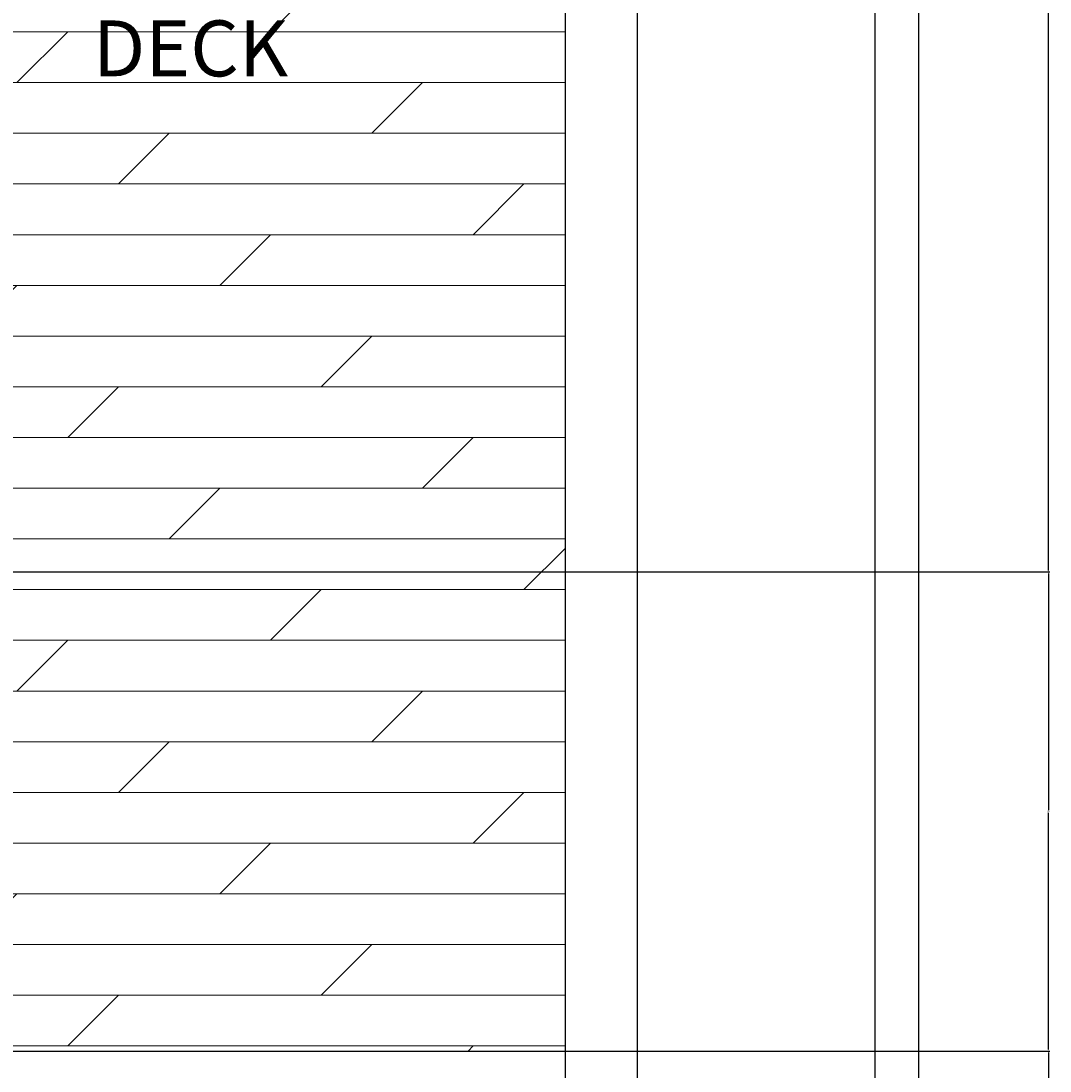
# Model space of a CAD drawing. Units: inches. Extents: x 84 to 1044, y -280 to 906.
# Tile 48 of 105: x 915 to 1044, y 29 to 160. Entities that reach past the tile are written whole.
import ezdxf

# ---------------------------------------------------------------- set-up
doc = ezdxf.new("R2010")
doc.units = ezdxf.units.IN
for name, color, linetype, lineweight in [('A-ANNO-DIMS', 2, 'Continuous', 18), ('A-ANNO-TTLB', 7, 'Continuous', 25), ('A-AREA-IDEN', 7, 'Continuous', 13), ('C-PROP', 7, 'Continuous', 25), ('L-POOL', 151, 'Continuous', 25)]:
    doc.layers.add(name, color=color, linetype=linetype, lineweight=lineweight)
doc.layers.add('A-FLOR-PATT', color=251, linetype='Continuous', lineweight=9, true_color=0x705861)
doc.styles.add('1-100DIM', font='txt', dxfattribs={"height": 0.3})
doc.styles.get("Standard").update_dxf_attribs({"font": 'arial.ttf'})
doc.dimstyles.get("Standard").update_dxf_attribs({"dimtxt": 0.18, "dimasz": 0.18, "dimexe": 0.18, "dimexo": 0.0625, "dimgap": 0.09, "dimtad": 0, "dimtih": 1, "dimtoh": 1, "dimdec": 4, "dimzin": 0, "dimdsep": 46, "dimtxsty": 'Standard', "dimcen": 0.09, "dimadec": 0, "dimazin": 0, "dimtfac": 1, "dimtdec": 4, "dimtofl": 0, "dimtmove": 0, "dimatfit": 3, "dimfxl": 1, "dimtolj": 1, "dimtzin": 0, "dimarcsym": 0})

# ---------------------------------------------------------------- blocks, each defined once
blk = doc.blocks.new('*D63')
at = {"layer": 'A-ANNO-DIMS', "color": 0, "lineweight": -2, "transparency": 16777216}
for p, q in [((833.14, 709.12), (1043.77, 709.12)), ((1043.59, 708.94), (1043.59, 400.3)), ((1043.59, 91.3), (1043.59, 399.94)), ((896.14, 91.12), (1043.77, 91.12))]:
    blk.add_line(p, q, dxfattribs=at)
at = {"layer": 'A-ANNO-DIMS', "color": 0, "transparency": 16777216}
for points in [[(1043.56, 708.94), (1043.62, 708.94), (1043.59, 709.12)], [(1043.56, 91.3), (1043.62, 91.3), (1043.59, 91.12)]]:
    blk.add_solid(points, dxfattribs=at)
at = {"layer": 'Defpoints', "color": 0, "transparency": 16777216}
for p in [(833.07, 709.12), (1043.59, 709.12), (896.07, 91.12)]:
    blk.add_point(p, dxfattribs=at)
at = {"layer": 'A-ANNO-DIMS', "color": 0, "transparency": 16777216, "insert": (1043.59, 400.12), "char_height": 0.18, "attachment_point": 5}
blk.add_mtext('\\A1;618', dxfattribs=at)
blk = doc.blocks.new('*D68')
at = {"layer": 'A-ANNO-DIMS', "color": 0, "lineweight": -2, "transparency": 16777216}
for p, q in [((983.14, 31.12), (1043.77, 31.12)), ((1043.59, 30.94), (1043.59, -16.7)), ((1043.59, -64.7), (1043.59, -17.06)), ((983.14, -64.88), (1043.77, -64.88))]:
    blk.add_line(p, q, dxfattribs=at)
at = {"layer": 'A-ANNO-DIMS', "color": 0, "transparency": 16777216}
for points in [[(1043.56, 30.94), (1043.62, 30.94), (1043.59, 31.12)], [(1043.56, -64.7), (1043.62, -64.7), (1043.59, -64.88)]]:
    blk.add_solid(points, dxfattribs=at)
at = {"layer": 'Defpoints', "color": 0, "transparency": 16777216}
for p in [(983.07, 31.12), (1043.59, 31.12), (983.07, -64.88)]:
    blk.add_point(p, dxfattribs=at)
at = {"layer": 'A-ANNO-DIMS', "color": 0, "transparency": 16777216, "insert": (1043.59, -16.88), "char_height": 0.18, "attachment_point": 5}
blk.add_mtext('\\A1;96', dxfattribs=at)
blk = doc.blocks.new('*D69')
at = {"layer": 'A-ANNO-DIMS', "color": 0, "lineweight": -2, "transparency": 16777216}
for p, q in [((896.14, 91.12), (1043.77, 91.12)), ((1043.59, 90.94), (1043.59, 61.3)), ((1043.59, 31.3), (1043.59, 60.94)), ((983.14, 31.12), (1043.77, 31.12))]:
    blk.add_line(p, q, dxfattribs=at)
at = {"layer": 'A-ANNO-DIMS', "color": 0, "transparency": 16777216}
for points in [[(1043.56, 90.94), (1043.62, 90.94), (1043.59, 91.12)], [(1043.56, 31.3), (1043.62, 31.3), (1043.59, 31.12)]]:
    blk.add_solid(points, dxfattribs=at)
at = {"layer": 'Defpoints', "color": 0, "transparency": 16777216}
for p in [(896.07, 91.12), (983.07, 31.12), (1043.59, 31.12)]:
    blk.add_point(p, dxfattribs=at)
at = {"layer": 'A-ANNO-DIMS', "color": 0, "transparency": 16777216, "insert": (1043.59, 61.12), "char_height": 0.18, "attachment_point": 5}
blk.add_mtext('\\A1;60', dxfattribs=at)

msp = doc.modelspace()

# ---------------------------------------------------------------- hatches: boundary and pattern name
at = {"layer": 'A-FLOR-PATT', "transparency": 33554597}
h = msp.add_hatch(dxfattribs=at)
h.set_pattern_fill('DOLMIT', color=256)
h.paths.add_polyline_path([(983.074, 265.12), (896.074, 265.12), (896.074, 91.12), (887.074, 91.12), (887.074, 31.12), (983.074, 31.12)])

# ---------------------------------------------------------------- linework, layer by layer
at = {"layer": 'A-ANNO-TTLB'}
for points in [[(101.1, 905.916), (1027.308, 905.916), (1027.308, -279.764), (101.1, -279.764)], [(106.576, 900.439), (1021.832, 900.439), (1021.832, -274.288), (106.576, -274.288)]]:
    msp.add_lwpolyline(points, close=True, dxfattribs=at)
at = {"layer": 'C-PROP'}
for points in [[(143.179, -121.88), (134.179, -121.88), (134.179, 856.12), (992.074, 856.12), (992.074, -121.88), (624.574, -121.88)], [(143.179, -112.88), (143.179, 847.12), (983.074, 847.12), (983.074, -112.88), (624.574, -112.88)]]:
    msp.add_lwpolyline(points, dxfattribs=at)
at = {"layer": 'L-POOL'}
msp.add_lwpolyline([(791.074, 31.12), (983.074, 31.12), (983.074, -64.88), (791.074, -64.88)], close=True, dxfattribs=at)

# ---------------------------------------------------------------- texts
at = {"layer": 'A-AREA-IDEN', "insert": (915.356, 160.191), "char_height": 7, "attachment_point": 1, "style": '1-100DIM'}
msp.add_mtext_dynamic_manual_height_columns('{\\f@Malgun Gothic|b0|i0|c0|p34;    DECK }', width=51.07953, gutter_width=15.851, heights=[0], dxfattribs=at)

# ---------------------------------------------------------------- dimensions: what is measured, and where the dimension line sits
at = {"layer": 'A-ANNO-DIMS'}
for base, p1, p2, picture, middle in [((1043.588, 709.12), (896.074, 91.12), (833.074, 709.12), '*D63', (1043.588, 400.12)), ((1043.588, 31.12), (896.074, 91.12), (983.074, 31.12), '*D69', (1043.588, 61.12)), ((1043.588, 31.12), (983.074, -64.88), (983.074, 31.12), '*D68', (1043.588, -16.88))]:
    dim = msp.add_linear_dim(base=base, p1=p1, p2=p2, angle=90, dimstyle='Standard', override={"dimdec": 0, "dimlfac": 1, "dimrnd": 0, "dimzin": 0, "dimdsep": 46, "dimlunit": 2}, dxfattribs=at)
    dim.commit()
    dim.dimension.update_dxf_attribs({"geometry": picture, "text_midpoint": middle})

doc.saveas('drawing.dxf')
